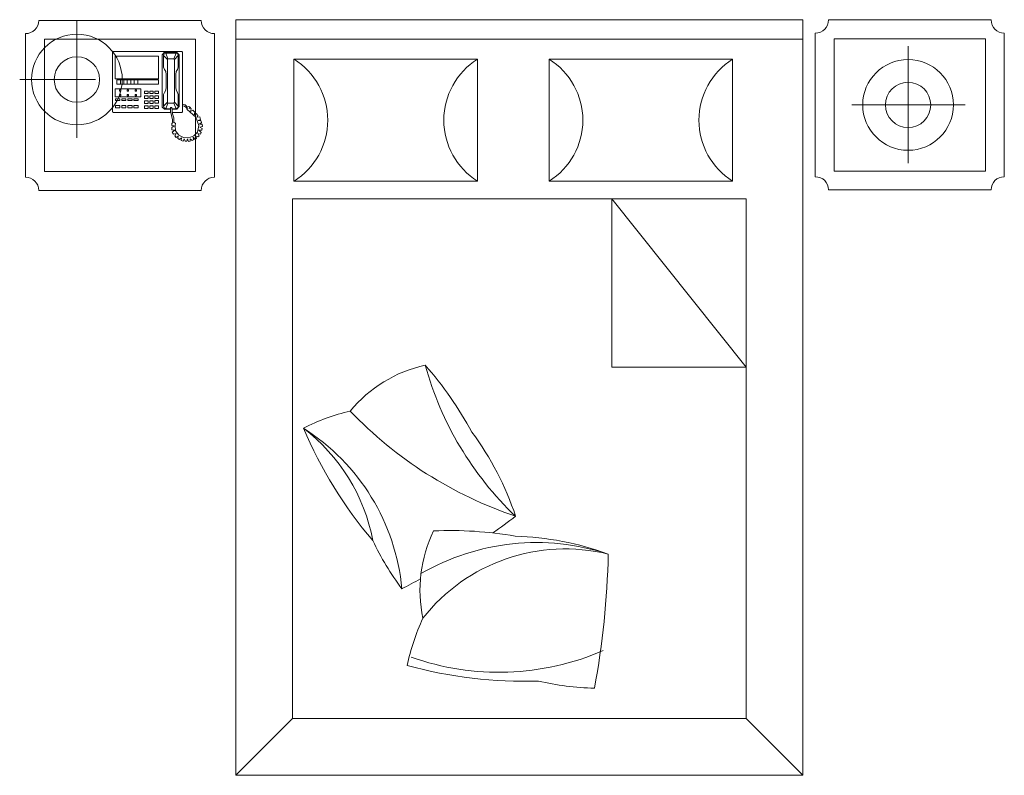
# Model space of a CAD drawing. Units: inches. Extents: x -108 to 1456, y -102 to 617.
# Tile 8 of 8: x 1374 to 1456, y -102 to -39. Entities that reach past the tile are written whole.
import ezdxf

# ---------------------------------------------------------------- set-up
doc = ezdxf.new("R2010")
doc.units = ezdxf.units.IN
doc.layers.add('A-FURN', color=8, linetype='Continuous', lineweight=18)

# ---------------------------------------------------------------- blocks, each defined once
blk = doc.blocks.new('A$C50B66110')
for p, q in [((0.0503, 1.9981), (0.4803, 1.9981)), ((0.1513, 1.6871), (0.1513, 1.9967)), ((0.5716, 1.9488), (0.5716, 2)), ((0.5716, 2), (2.0719, 2)), ((2.0719, 1.9488), (2.0719, 2)), ((2.5701, 1.9993), (2.1401, 1.9993)), ((0.0153, 1.9631), (0.0153, 1.5831)), ((0.5153, 1.9631), (0.5153, 1.5831)), ((2.1051, 1.9643), (2.1051, 1.5843)), ((2.6051, 1.9643), (2.6051, 1.5843)), ((0.0653, 1.9481), (0.0653, 1.5981)), ((0.0653, 1.9481), (0.4653, 1.9481)), ((0.4653, 1.9481), (0.4653, 1.5981)), ((2.0719, 1.9488), (0.5716, 1.9488)), ((0.5716, 1.9488), (0.5716, 0)), ((2.0719, 0), (2.0719, 1.9488)), ((2.1551, 1.9493), (2.1551, 1.5993)), ((2.5551, 1.9493), (2.1551, 1.9493)), ((2.3505, 1.62), (2.3505, 1.9295)), ((2.5551, 1.9493), (2.5551, 1.5993)), ((0.7257, 1.5725), (0.7257, 1.8954)), ((0.7257, 1.8954), (1.2113, 1.8954)), ((1.2113, 1.8954), (1.2113, 1.5725)), ((1.4007, 1.5725), (1.4007, 1.8954)), ((1.4007, 1.8954), (1.8863, 1.8954)), ((1.8863, 1.8954), (1.8863, 1.5725)), ((0, 1.8416), (0.2001, 1.8416)), ((2.5018, 1.7744), (2.2017, 1.7744)), ((0.0653, 1.5981), (0.4653, 1.5981)), ((2.5551, 1.5993), (2.1551, 1.5993)), ((1.2113, 1.5725), (0.7257, 1.5725)), ((1.8863, 1.5725), (1.4007, 1.5725)), ((0.0503, 1.5481), (0.4803, 1.5481)), ((2.5701, 1.5493), (2.1401, 1.5493)), ((1.5665, 1.5254), (1.5665, 1.0802)), ((1.5665, 1.5254), (1.9219, 1.0802)), ((1.9219, 1.0802), (1.5665, 1.0802)), ((0.5716, 0), (0.7216, 0.15)), ((2.0719, 0), (1.9219, 0.15)), ((0.5716, 0), (2.0719, 0))]:
    blk.add_line(p, q)
at = {"linetype": 'ByBlock'}
for p, q in [((0.2481, 1.9162), (0.2458, 1.9139)), ((0.2458, 1.9139), (0.2458, 1.7562)), ((0.2481, 1.9162), (0.4287, 1.9162)), ((0.2526, 1.9036), (0.2526, 1.8431)), ((0.3669, 1.9036), (0.2526, 1.9036)), ((0.3669, 1.8431), (0.3669, 1.9036)), ((0.3772, 1.9071), (0.3818, 1.9128)), ((0.3772, 1.7688), (0.3772, 1.9071)), ((0.3818, 1.9094), (0.3807, 1.9048)), ((0.3807, 1.9048), (0.3807, 1.8739)), ((0.3807, 1.9048), (0.3909, 1.8945)), ((0.3818, 1.9128), (0.4161, 1.9128)), ((0.3864, 1.9116), (0.3818, 1.9094)), ((0.3921, 1.8968), (0.3864, 1.9116)), ((0.3864, 1.9116), (0.4138, 1.9116)), ((0.4081, 1.8968), (0.4138, 1.9116)), ((0.4195, 1.9048), (0.4092, 1.8945)), ((0.4138, 1.9116), (0.4184, 1.9094)), ((0.4161, 1.9128), (0.4218, 1.9071)), ((0.4184, 1.9094), (0.4195, 1.9048)), ((0.4195, 1.9048), (0.4195, 1.8739)), ((0.4218, 1.9071), (0.4218, 1.7699)), ((0.4287, 1.9162), (0.4309, 1.9139)), ((0.4309, 1.9139), (0.4309, 1.7562)), ((0.3909, 1.8945), (0.3921, 1.8968)), ((0.3909, 1.8431), (0.3909, 1.8945)), ((0.4081, 1.8968), (0.3921, 1.8968)), ((0.4092, 1.8945), (0.4081, 1.8968)), ((0.4092, 1.8431), (0.4092, 1.8945)), ((0.3807, 1.8739), (0.3829, 1.8682)), ((0.3829, 1.8682), (0.3864, 1.8625)), ((0.3864, 1.8625), (0.3875, 1.8545)), ((0.3875, 1.8545), (0.3875, 1.8431)), ((0.4138, 1.8625), (0.4127, 1.8545)), ((0.4127, 1.8545), (0.4127, 1.8431)), ((0.4172, 1.8682), (0.4138, 1.8625)), ((0.4195, 1.8739), (0.4172, 1.8682)), ((0.2526, 1.8431), (0.3669, 1.8431)), ((0.2572, 1.8408), (0.2572, 1.8294)), ((0.3669, 1.8408), (0.2572, 1.8408)), ((0.2572, 1.8294), (0.3669, 1.8294)), ((0.2664, 1.8408), (0.2664, 1.8294)), ((0.2755, 1.8408), (0.2755, 1.8294)), ((0.2846, 1.8408), (0.2846, 1.8294)), ((0.2938, 1.8408), (0.2938, 1.8294)), ((0.3029, 1.8408), (0.3029, 1.8294)), ((0.3121, 1.8408), (0.3121, 1.8294)), ((0.3669, 1.8294), (0.3669, 1.8408)), ((0.3875, 1.8214), (0.3875, 1.8431)), ((0.3909, 1.8431), (0.3909, 1.7813)), ((0.4092, 1.8431), (0.4092, 1.7813)), ((0.4127, 1.8214), (0.4127, 1.8431)), ((0.3201, 1.8168), (0.2526, 1.8168)), ((0.2526, 1.8168), (0.2526, 1.7962)), ((0.2675, 1.8145), (0.2641, 1.8145)), ((0.2641, 1.8145), (0.2641, 1.8111)), ((0.2641, 1.8111), (0.2675, 1.8111)), ((0.2641, 1.8019), (0.2641, 1.7985)), ((0.2675, 1.8019), (0.2641, 1.8019)), ((0.2641, 1.7985), (0.2675, 1.7985)), ((0.2675, 1.8111), (0.2675, 1.8145)), ((0.2675, 1.7985), (0.2675, 1.8019)), ((0.2846, 1.8145), (0.2846, 1.8111)), ((0.2881, 1.8145), (0.2846, 1.8145)), ((0.2846, 1.8111), (0.2881, 1.8111)), ((0.2846, 1.8019), (0.2846, 1.7985)), ((0.2881, 1.8019), (0.2846, 1.8019)), ((0.2846, 1.7985), (0.2881, 1.7985)), ((0.2881, 1.8111), (0.2881, 1.8145)), ((0.2881, 1.7985), (0.2881, 1.8019)), ((0.3052, 1.8145), (0.3052, 1.8111)), ((0.3086, 1.8145), (0.3052, 1.8145)), ((0.3052, 1.8111), (0.3086, 1.8111)), ((0.3052, 1.8019), (0.3052, 1.7985)), ((0.3086, 1.8019), (0.3052, 1.8019)), ((0.3052, 1.7985), (0.3086, 1.7985)), ((0.3086, 1.8111), (0.3086, 1.8145)), ((0.3086, 1.7985), (0.3086, 1.8019)), ((0.3201, 1.7962), (0.3201, 1.8168)), ((0.3304, 1.8111), (0.3395, 1.8111)), ((0.3304, 1.8042), (0.3304, 1.8111)), ((0.3395, 1.8042), (0.3304, 1.8042)), ((0.3304, 1.7985), (0.3395, 1.7985)), ((0.3304, 1.7916), (0.3304, 1.7985)), ((0.3395, 1.8111), (0.3395, 1.8042)), ((0.3395, 1.7985), (0.3395, 1.7916)), ((0.3441, 1.8042), (0.3441, 1.8111)), ((0.3441, 1.8111), (0.3532, 1.8111)), ((0.3532, 1.8042), (0.3441, 1.8042)), ((0.3441, 1.7985), (0.3532, 1.7985)), ((0.3441, 1.7916), (0.3441, 1.7985)), ((0.3532, 1.8111), (0.3532, 1.8042)), ((0.3532, 1.7985), (0.3532, 1.7916)), ((0.3578, 1.8111), (0.3669, 1.8111)), ((0.3578, 1.8042), (0.3578, 1.8111)), ((0.3669, 1.8042), (0.3578, 1.8042)), ((0.3578, 1.7985), (0.3669, 1.7985)), ((0.3578, 1.7916), (0.3578, 1.7985)), ((0.3669, 1.8111), (0.3669, 1.8042)), ((0.3669, 1.7985), (0.3669, 1.7916)), ((0.3807, 1.8019), (0.3829, 1.8076)), ((0.3807, 1.7711), (0.3807, 1.8019)), ((0.3829, 1.8076), (0.3864, 1.8134)), ((0.3864, 1.8134), (0.3875, 1.8214)), ((0.4138, 1.8134), (0.4127, 1.8214)), ((0.4172, 1.8076), (0.4138, 1.8134)), ((0.4195, 1.8019), (0.4172, 1.8076)), ((0.4195, 1.7711), (0.4195, 1.8019)), ((0.2526, 1.7962), (0.3201, 1.7962)), ((0.2652, 1.7905), (0.2538, 1.7905)), ((0.2538, 1.7905), (0.2538, 1.7859)), ((0.2538, 1.7859), (0.2652, 1.7859)), ((0.2538, 1.7665), (0.2538, 1.7733)), ((0.2538, 1.7733), (0.2652, 1.7733)), ((0.2652, 1.7859), (0.2652, 1.7905)), ((0.2652, 1.7733), (0.2652, 1.7665)), ((0.2812, 1.7905), (0.2698, 1.7905)), ((0.2698, 1.7905), (0.2698, 1.7859)), ((0.2698, 1.7859), (0.2812, 1.7859)), ((0.2698, 1.7665), (0.2698, 1.7733)), ((0.2698, 1.7733), (0.2812, 1.7733)), ((0.2812, 1.7859), (0.2812, 1.7905)), ((0.2812, 1.7733), (0.2812, 1.7665)), ((0.2972, 1.7905), (0.2858, 1.7905)), ((0.2858, 1.7905), (0.2858, 1.7859)), ((0.2858, 1.7859), (0.2972, 1.7859)), ((0.2858, 1.7665), (0.2858, 1.7733)), ((0.2858, 1.7733), (0.2972, 1.7733)), ((0.2972, 1.7859), (0.2972, 1.7905)), ((0.2972, 1.7733), (0.2972, 1.7665)), ((0.3018, 1.7905), (0.3018, 1.7859)), ((0.3132, 1.7905), (0.3018, 1.7905)), ((0.3018, 1.7859), (0.3132, 1.7859)), ((0.3018, 1.7733), (0.3132, 1.7733)), ((0.3018, 1.7665), (0.3018, 1.7733)), ((0.3132, 1.7859), (0.3132, 1.7905)), ((0.3132, 1.7733), (0.3132, 1.7665)), ((0.3395, 1.7916), (0.3304, 1.7916)), ((0.3304, 1.7779), (0.3304, 1.7848)), ((0.3304, 1.7848), (0.3395, 1.7848)), ((0.3395, 1.7779), (0.3304, 1.7779)), ((0.3304, 1.7722), (0.3395, 1.7722)), ((0.3304, 1.7653), (0.3304, 1.7722)), ((0.3395, 1.7848), (0.3395, 1.7779)), ((0.3395, 1.7722), (0.3395, 1.7653)), ((0.3532, 1.7916), (0.3441, 1.7916)), ((0.3441, 1.7779), (0.3441, 1.7848)), ((0.3441, 1.7848), (0.3532, 1.7848)), ((0.3532, 1.7779), (0.3441, 1.7779)), ((0.3441, 1.7722), (0.3532, 1.7722)), ((0.3441, 1.7653), (0.3441, 1.7722)), ((0.3532, 1.7848), (0.3532, 1.7779)), ((0.3532, 1.7722), (0.3532, 1.7653)), ((0.3669, 1.7916), (0.3578, 1.7916)), ((0.3578, 1.7791), (0.3578, 1.7859)), ((0.3578, 1.7859), (0.3669, 1.7859)), ((0.3669, 1.7791), (0.3578, 1.7791)), ((0.3578, 1.7653), (0.3578, 1.7722)), ((0.3578, 1.7722), (0.3669, 1.7722)), ((0.3669, 1.7859), (0.3669, 1.7791)), ((0.3669, 1.7722), (0.3669, 1.7653)), ((0.3807, 1.7711), (0.3909, 1.7813)), ((0.3921, 1.7791), (0.3864, 1.7642)), ((0.3909, 1.7813), (0.3921, 1.7791)), ((0.4081, 1.7791), (0.3921, 1.7791)), ((0.4092, 1.7813), (0.4081, 1.7791)), ((0.4081, 1.7791), (0.4138, 1.7642)), ((0.4195, 1.7711), (0.4092, 1.7813)), ((0.4378, 1.7742), (0.4309, 1.7768)), ((0.4309, 1.7722), (0.436, 1.7708)), ((0.441, 1.771), (0.4378, 1.7742)), ((0.2458, 1.7562), (0.2481, 1.7539)), ((0.4, 1.7539), (0.2481, 1.7539)), ((0.2652, 1.7665), (0.2538, 1.7665)), ((0.2812, 1.7665), (0.2698, 1.7665)), ((0.2972, 1.7665), (0.2858, 1.7665)), ((0.3132, 1.7665), (0.3018, 1.7665)), ((0.3395, 1.7653), (0.3304, 1.7653)), ((0.3532, 1.7653), (0.3441, 1.7653)), ((0.3669, 1.7653), (0.3578, 1.7653)), ((0.3829, 1.7631), (0.3772, 1.7688)), ((0.3818, 1.7665), (0.3807, 1.7711)), ((0.3864, 1.7642), (0.3818, 1.7665)), ((0.399, 1.7631), (0.3829, 1.7631)), ((0.3864, 1.7642), (0.399, 1.7642)), ((0.4024, 1.7676), (0.3989, 1.7676)), ((0.3989, 1.7676), (0.3991, 1.7578)), ((0.3991, 1.7578), (0.4019, 1.7462)), ((0.4019, 1.7462), (0.4047, 1.7353)), ((0.403, 1.7585), (0.4024, 1.7676)), ((0.4026, 1.7642), (0.4138, 1.7642)), ((0.4161, 1.7631), (0.4027, 1.7631)), ((0.4047, 1.7511), (0.403, 1.7585)), ((0.4287, 1.7539), (0.404, 1.7539)), ((0.4074, 1.7402), (0.4047, 1.7511)), ((0.4138, 1.7642), (0.4184, 1.7665)), ((0.4218, 1.7699), (0.4161, 1.7631)), ((0.4184, 1.7665), (0.4195, 1.7711)), ((0.4309, 1.7562), (0.4287, 1.7539)), ((0.436, 1.7708), (0.4406, 1.7672)), ((0.4406, 1.7672), (0.4418, 1.7656)), ((0.4434, 1.7688), (0.441, 1.771)), ((0.4443, 1.7658), (0.4418, 1.7633)), ((0.4418, 1.7656), (0.4443, 1.7658)), ((0.4418, 1.7633), (0.4511, 1.7551)), ((0.4477, 1.7704), (0.4434, 1.7688)), ((0.4497, 1.7684), (0.4477, 1.7704)), ((0.4481, 1.765), (0.4497, 1.7684)), ((0.4509, 1.7672), (0.4481, 1.765)), ((0.4539, 1.764), (0.4509, 1.7672)), ((0.4511, 1.7551), (0.4662, 1.7422)), ((0.4515, 1.7573), (0.4539, 1.764)), ((0.4577, 1.7605), (0.4515, 1.7573)), ((0.463, 1.7555), (0.4577, 1.7605)), ((0.4618, 1.7482), (0.463, 1.7555)), ((0.467, 1.7515), (0.4618, 1.7482)), ((0.4714, 1.7468), (0.467, 1.7515)), ((0.4696, 1.7418), (0.4714, 1.7468)), ((0.4026, 1.7254), (0.4021, 1.7198)), ((0.4021, 1.7198), (0.4088, 1.7187)), ((0.4051, 1.7279), (0.4026, 1.7254)), ((0.4047, 1.7353), (0.4044, 1.7293)), ((0.4044, 1.7293), (0.4051, 1.7279)), ((0.4081, 1.7346), (0.4074, 1.7402)), ((0.4079, 1.7286), (0.4081, 1.7346)), ((0.4121, 1.7256), (0.4079, 1.7286)), ((0.4111, 1.7203), (0.4121, 1.7256)), ((0.4123, 1.7057), (0.4111, 1.7203)), ((0.4664, 1.7418), (0.4741, 1.72)), ((0.4766, 1.7425), (0.4697, 1.7418)), ((0.4741, 1.72), (0.4708, 1.7027)), ((0.472, 1.733), (0.4787, 1.7356)), ((0.4794, 1.7332), (0.472, 1.733)), ((0.4761, 1.7233), (0.481, 1.7279)), ((0.4824, 1.7233), (0.4761, 1.7233)), ((0.4787, 1.7356), (0.4766, 1.7425)), ((0.481, 1.7279), (0.4794, 1.7332)), ((0.4835, 1.7175), (0.4824, 1.7233)), ((0.4088, 1.7187), (0.4023, 1.7147)), ((0.4023, 1.7147), (0.4028, 1.7085)), ((0.4028, 1.7085), (0.4102, 1.7078)), ((0.4102, 1.7078), (0.4037, 1.7027)), ((0.4037, 1.7027), (0.4067, 1.6974)), ((0.4067, 1.6974), (0.4137, 1.6988)), ((0.4137, 1.6988), (0.4104, 1.6923)), ((0.4211, 1.6946), (0.4123, 1.7057)), ((0.4333, 1.6881), (0.4211, 1.6946)), ((0.4708, 1.7027), (0.4606, 1.6927)), ((0.4745, 1.6925), (0.4713, 1.6988)), ((0.4713, 1.6988), (0.478, 1.6967)), ((0.4743, 1.7075), (0.4815, 1.7073)), ((0.4798, 1.7013), (0.4743, 1.7075)), ((0.4764, 1.7154), (0.4835, 1.7175)), ((0.4824, 1.7119), (0.4764, 1.7154)), ((0.478, 1.6967), (0.4798, 1.7013)), ((0.4815, 1.7073), (0.4824, 1.7119)), ((0.4104, 1.6923), (0.4139, 1.6881)), ((0.4139, 1.6881), (0.4192, 1.692)), ((0.4192, 1.692), (0.4183, 1.6858)), ((0.4183, 1.6858), (0.4227, 1.683)), ((0.4227, 1.683), (0.4283, 1.6876)), ((0.4283, 1.6876), (0.4276, 1.68)), ((0.4276, 1.68), (0.4324, 1.6786)), ((0.4324, 1.6786), (0.4354, 1.6849)), ((0.4472, 1.6869), (0.4333, 1.6881)), ((0.4354, 1.6849), (0.4382, 1.6786)), ((0.4382, 1.6786), (0.4421, 1.6782)), ((0.4421, 1.6782), (0.4437, 1.6849)), ((0.4437, 1.6849), (0.4463, 1.6775)), ((0.4463, 1.6775), (0.4507, 1.6786)), ((0.4606, 1.6927), (0.4472, 1.6869)), ((0.4507, 1.6786), (0.4509, 1.6849)), ((0.4509, 1.6849), (0.4562, 1.6802)), ((0.4562, 1.6802), (0.4599, 1.6821)), ((0.4592, 1.689), (0.4641, 1.683)), ((0.4599, 1.6821), (0.4592, 1.689)), ((0.4641, 1.683), (0.4678, 1.6863)), ((0.465, 1.6925), (0.4715, 1.6897)), ((0.4678, 1.6863), (0.465, 1.6925)), ((0.4715, 1.6897), (0.4745, 1.6925)), ((0.7216, 1.5254), (1.9219, 1.5254)), ((0.7216, 1.5254), (0.7216, 0.15)), ((1.9219, 0.15), (1.9219, 1.5254)), ((0.7216, 0.15), (1.9219, 0.15))]:
    blk.add_line(p, q, dxfattribs=at)
for centre, radius in [((0.1513, 1.8416), 0.12), ((0.1513, 1.8416), 0.06), ((2.3505, 1.7744), 0.12), ((2.3505, 1.7744), 0.06)]:
    blk.add_circle(centre, radius)
for centre, radius, start, end in [((0.0153, 1.9981), 0.035, 270, 0), ((0.5153, 1.9981), 0.035, 180, 270), ((2.1051, 1.9993), 0.035, 270, 0), ((2.6051, 1.9993), 0.035, 180, 270), ((0.6244, 1.734), 0.1906, 302.1202, 57.8798), ((1.3126, 1.734), 0.1906, 122.1202, 237.8798), ((1.2994, 1.734), 0.1906, 302.1202, 57.8798), ((1.9876, 1.734), 0.1906, 122.1202, 237.8798), ((0.0153, 1.5481), 0.035, 0, 90), ((0.5153, 1.5481), 0.035, 90, 180), ((2.1051, 1.5493), 0.035, 0, 90), ((2.6051, 1.5493), 0.035, 90, 180), ((1.1502, 0.7366), 0.3575, 102.4782, 140.4625), ((0.328, 0.4368), 0.9879, 28.4971, 41.0566), ((1.9117, 1.3157), 0.8697, 195.336, 226.4193), ((0.9996, 0.4307), 0.548, 103.2034, 117.0362), ((1.656, 1.7093), 1.0798, 223.6306, 251.4288), ((0.4482, 0.4408), 0.5655, 5.3391, 57.6895), ((1.8226, 1.3753), 1.1652, 203.0642, 220.3209), ((0.4548, 0.5307), 0.4879, 10.6986, 52.6864), ((0.5648, 0.4378), 0.7874, 18.3527, 36.6851), ((-0.0179, 2.4352), 2.1977, 305.2966, 307.2418), ((1.4166, 0.4903), 0.3575, 154.0418, 192.0262), ((1.1403, -0.3401), 0.9879, 80.0607, 92.6202), ((1.2867, -0.154), 0.7874, 69.9163, 88.2487), ((1.5981, 0.9345), 0.734, 205.259, 216.9351), ((1.3672, 0.0075), 0.6085, 71.81, 120.1351), ((1.4431, 0.1219), 0.4774, 76.1849, 142.0017), ((-0.6401, 0.6314), 2.1977, 349.4884, 358.8054), ((-0.0179, 2.4352), 2.1977, 297.9248, 299.3793), ((1.5626, 0.1822), 0.548, 154.767, 168.5998), ((1.2678, 0.9611), 0.6885, 250.2936, 293.6414), ((1.3343, 1.4141), 1.1652, 254.6278, 271.8845), ((1.5399, 0.9642), 0.734, 256.8226, 268.4988)]:
    blk.add_arc(centre, radius, start, end)

msp = doc.modelspace()

# ---------------------------------------------------------------- block references
at = {"layer": 'A-FURN', "xscale": 31.47959221109753, "yscale": 31.47959221109753, "zscale": 31.47959221109753}
msp.add_blockref('A$C50B66110', (1373.6098, -101.662), dxfattribs=at)

doc.saveas('drawing.dxf')
